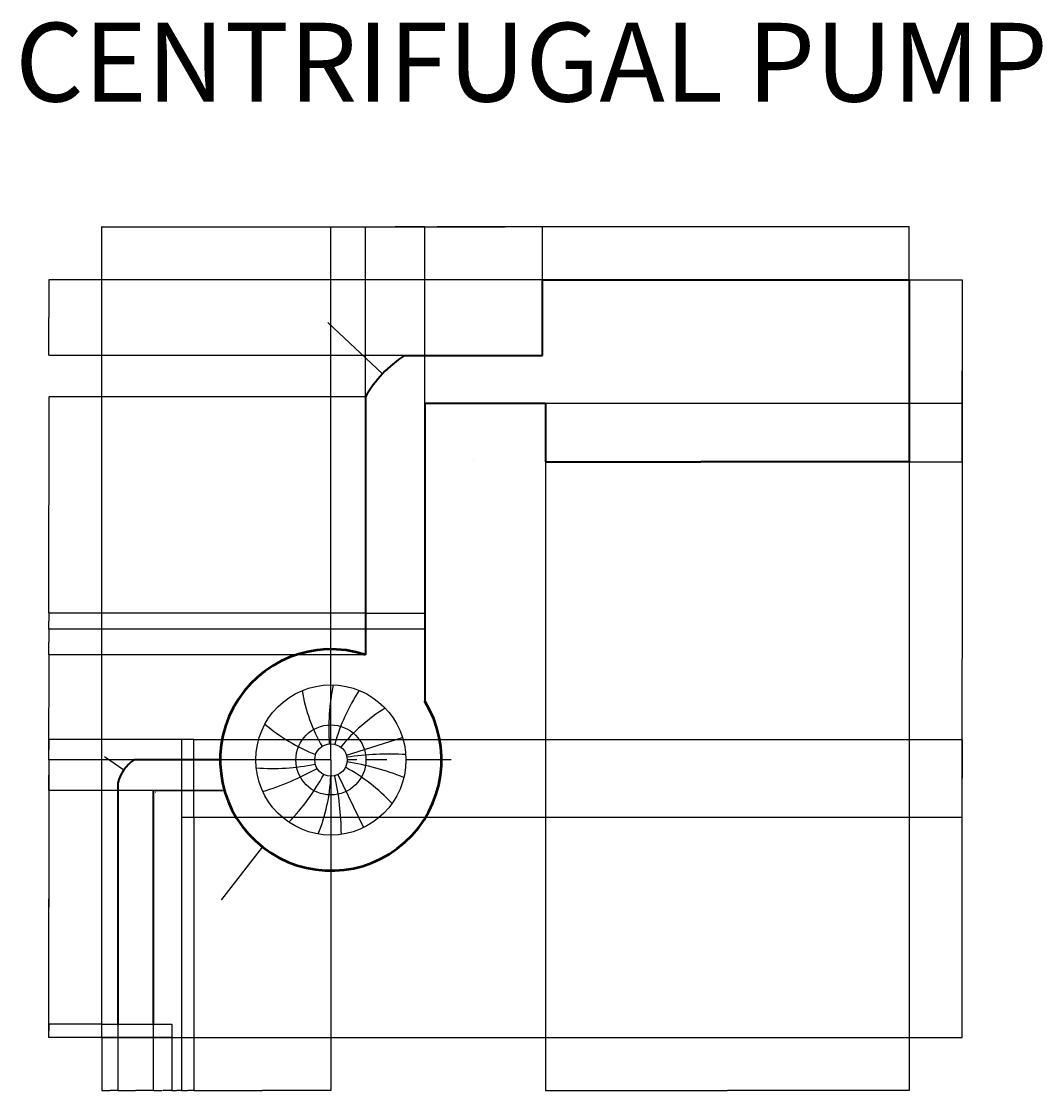
# Model space of a CAD drawing. Units: millimetres. Extents: x 1905 to 3850, y 1033 to 3069.
import ezdxf

# ---------------------------------------------------------------- set-up
doc = ezdxf.new("R2010")
doc.units = ezdxf.units.MM
for name, color, linetype, lineweight in [('A-ANNO-DIMS', 2, 'Continuous', 18), ('M-ANNO-TEXT', 7, 'Continuous', 25), ('M-EQPM-CASG', 7, 'Continuous', 50), ('M-EQPM-IMPL', 4, 'Continuous', 25), ('P-EQPM-TANK', 5, 'Continuous', 35), ('P-PIPE', 3, 'Continuous', 35), ('P-PIPE-FLNG', 6, 'Continuous', 25)]:
    doc.layers.add(name, color=color, linetype=linetype, lineweight=lineweight)
doc.styles.get("Standard").update_dxf_attribs({"font": 'arial.ttf'})
doc.dimstyles.get("Standard").update_dxf_attribs({"dimtxt": 0.18, "dimasz": 0.18, "dimexe": 0.18, "dimexo": 0.0625, "dimgap": 0.09, "dimtad": 0, "dimtih": 1, "dimtoh": 1, "dimdec": 4, "dimzin": 0, "dimdsep": 46, "dimtxsty": 'Standard', "dimcen": 0.09, "dimadec": 0, "dimazin": 0, "dimtfac": 1, "dimtdec": 4, "dimtofl": 0, "dimtmove": 0, "dimatfit": 3, "dimfxl": 1, "dimtolj": 1, "dimtzin": 0, "dimarcsym": 0})

# ---------------------------------------------------------------- blocks, each defined once
blk = doc.blocks.new('*D1')
at = {"layer": 'A-ANNO-DIMS', "color": 0, "lineweight": -2, "transparency": 16777216}
for p, q in [((2058, 1134.2), (2058, 2678.4)), ((2058.1, 2678.2), (2826.3, 2678.2)), ((3595.5, 2678.2), (2827.3, 2678.2)), ((3595.6, 2577.3), (3595.6, 2678.4))]:
    blk.add_line(p, q, dxfattribs=at)
at = {"layer": 'A-ANNO-DIMS', "color": 0, "transparency": 16777216}
for points in [[(2058.1, 2678.3), (2058.1, 2678.2), (2058, 2678.2)], [(3595.5, 2678.3), (3595.5, 2678.2), (3595.6, 2678.2)]]:
    blk.add_solid(points, dxfattribs=at)
at = {"layer": 'Defpoints', "color": 0, "transparency": 16777216}
for p in [(3595.6, 2678.2), (3595.6, 2577.2), (2058, 1134.2)]:
    blk.add_point(p, dxfattribs=at)
at = {"layer": 'A-ANNO-DIMS', "color": 0, "transparency": 16777216, "insert": (2826.8, 2678.2), "char_height": 0.18, "attachment_point": 5}
blk.add_mtext('\\A1;1537.7', dxfattribs=at)
blk = doc.blocks.new('*D2')
at = {"layer": 'A-ANNO-DIMS', "color": 0, "lineweight": -2, "transparency": 16777216}
for p, q in [((3595.7, 2577.2), (3696.8, 2577.2)), ((3696.6, 2577), (3696.6, 1855.9)), ((3696.6, 1134.3), (3696.6, 1855.5)), ((2058, 1134.2), (3696.8, 1134.2))]:
    blk.add_line(p, q, dxfattribs=at)
at = {"layer": 'A-ANNO-DIMS', "color": 0, "transparency": 16777216}
for points in [[(3696.6, 2577), (3696.7, 2577), (3696.6, 2577.2)], [(3696.6, 1134.3), (3696.7, 1134.3), (3696.6, 1134.2)]]:
    blk.add_solid(points, dxfattribs=at)
at = {"layer": 'Defpoints', "color": 0, "transparency": 16777216}
for p in [(3595.6, 2577.2), (3696.6, 2577.2), (2058, 1134.2)]:
    blk.add_point(p, dxfattribs=at)
at = {"layer": 'A-ANNO-DIMS', "color": 0, "transparency": 16777216, "insert": (3696.6, 1855.7), "char_height": 0.18, "attachment_point": 5}
blk.add_mtext('\\A1;1443', dxfattribs=at)
blk = doc.blocks.new('*D3')
at = {"layer": 'A-ANNO-DIMS', "color": 0, "lineweight": -2, "transparency": 16777216}
for p, q in [((3595.7, 2577.2), (3696.8, 2577.2)), ((3696.6, 2577), (3696.6, 2404.1)), ((3696.6, 2230.9), (3696.6, 2403.8)), ((3595.7, 2230.7), (3696.8, 2230.7))]:
    blk.add_line(p, q, dxfattribs=at)
at = {"layer": 'A-ANNO-DIMS', "color": 0, "transparency": 16777216}
for points in [[(3696.6, 2577), (3696.7, 2577), (3696.6, 2577.2)], [(3696.6, 2230.9), (3696.7, 2230.9), (3696.6, 2230.7)]]:
    blk.add_solid(points, dxfattribs=at)
at = {"layer": 'Defpoints', "color": 0, "transparency": 16777216}
for p in [(3595.6, 2577.2), (3696.6, 2577.2), (3595.6, 2230.7)]:
    blk.add_point(p, dxfattribs=at)
at = {"layer": 'A-ANNO-DIMS', "color": 0, "transparency": 16777216, "insert": (3696.6, 2404), "char_height": 0.18, "attachment_point": 5}
blk.add_mtext('\\A1;346.5', dxfattribs=at)
blk = doc.blocks.new('*D4')
at = {"layer": 'A-ANNO-DIMS', "color": 0, "lineweight": -2, "transparency": 16777216}
for p, q in [((2559.8, 2354.1), (2559.8, 2678.4)), ((2560, 2678.2), (2615.9, 2678.2)), ((2672.8, 2678.2), (2616.8, 2678.2)), ((2672.9, 2342), (2672.9, 2678.4))]:
    blk.add_line(p, q, dxfattribs=at)
at = {"layer": 'A-ANNO-DIMS', "color": 0, "transparency": 16777216}
for points in [[(2560, 2678.3), (2560, 2678.2), (2559.8, 2678.2)], [(2672.8, 2678.3), (2672.8, 2678.2), (2672.9, 2678.2)]]:
    blk.add_solid(points, dxfattribs=at)
at = {"layer": 'Defpoints', "color": 0, "transparency": 16777216}
for p in [(2672.9, 2678.2), (2559.8, 2354), (2672.9, 2341.9)]:
    blk.add_point(p, dxfattribs=at)
at = {"layer": 'A-ANNO-DIMS', "color": 0, "transparency": 16777216, "insert": (2616.4, 2678.2), "char_height": 0.18, "attachment_point": 5}
blk.add_mtext('\\A1;113.14', dxfattribs=at)
blk = doc.blocks.new('*D5')
at = {"layer": 'A-ANNO-DIMS', "color": 0, "lineweight": -2, "transparency": 16777216}
for p, q in [((2088.4, 1157.8), (2088.4, 1033)), ((2058, 1134.1), (2058, 1033)), ((2058.1, 1033.2), (2072.8, 1033.2)), ((2088.2, 1033.2), (2073.6, 1033.2))]:
    blk.add_line(p, q, dxfattribs=at)
at = {"layer": 'A-ANNO-DIMS', "color": 0, "transparency": 16777216}
for points in [[(2058.1, 1033.2), (2058.1, 1033.1), (2058, 1033.2)], [(2088.2, 1033.2), (2088.2, 1033.1), (2088.4, 1033.2)]]:
    blk.add_solid(points, dxfattribs=at)
at = {"layer": 'Defpoints', "color": 0, "transparency": 16777216}
for p in [(2088.4, 1157.9), (2058, 1134.2), (2088.4, 1033.2)]:
    blk.add_point(p, dxfattribs=at)
at = {"layer": 'A-ANNO-DIMS', "color": 0, "transparency": 16777216, "insert": (2073.2, 1033.2), "char_height": 0.18, "attachment_point": 5}
blk.add_mtext('\\A1;30.45', dxfattribs=at)
blk = doc.blocks.new('*D6')
at = {"layer": 'A-ANNO-DIMS', "color": 0, "lineweight": -2, "transparency": 16777216}
for p, q in [((2088.4, 1157.8), (2088.4, 1033)), ((2155.9, 1157.8), (2155.9, 1033)), ((2088.6, 1033.2), (2121.8, 1033.2)), ((2155.7, 1033.2), (2122.5, 1033.2))]:
    blk.add_line(p, q, dxfattribs=at)
at = {"layer": 'A-ANNO-DIMS', "color": 0, "transparency": 16777216}
for points in [[(2088.6, 1033.2), (2088.6, 1033.1), (2088.4, 1033.2)], [(2155.7, 1033.2), (2155.7, 1033.1), (2155.9, 1033.2)]]:
    blk.add_solid(points, dxfattribs=at)
at = {"layer": 'Defpoints', "color": 0, "transparency": 16777216}
for p in [(2088.4, 1157.9), (2155.9, 1157.9), (2155.9, 1033.2)]:
    blk.add_point(p, dxfattribs=at)
at = {"layer": 'A-ANNO-DIMS', "color": 0, "transparency": 16777216, "insert": (2122.1, 1033.2), "char_height": 0.18, "attachment_point": 5}
blk.add_mtext('\\A1;67.46', dxfattribs=at)
blk = doc.blocks.new('*D7')
at = {"layer": 'A-ANNO-DIMS', "color": 0, "lineweight": -2, "transparency": 16777216}
for p, q in [((2155.9, 1157.8), (2155.9, 1033)), ((2191.2, 1134.1), (2191.2, 1033)), ((2156.1, 1033.2), (2173.1, 1033.2)), ((2191, 1033.2), (2174, 1033.2))]:
    blk.add_line(p, q, dxfattribs=at)
at = {"layer": 'A-ANNO-DIMS', "color": 0, "transparency": 16777216}
for points in [[(2156.1, 1033.2), (2156.1, 1033.1), (2155.9, 1033.2)], [(2191, 1033.2), (2191, 1033.1), (2191.2, 1033.2)]]:
    blk.add_solid(points, dxfattribs=at)
at = {"layer": 'Defpoints', "color": 0, "transparency": 16777216}
for p in [(2155.9, 1157.9), (2191.2, 1134.2), (2191.2, 1033.2)]:
    blk.add_point(p, dxfattribs=at)
at = {"layer": 'A-ANNO-DIMS', "color": 0, "transparency": 16777216, "insert": (2173.5, 1033.2), "char_height": 0.18, "attachment_point": 5}
blk.add_mtext('\\A1;35.306', dxfattribs=at)
blk = doc.blocks.new('*D8')
at = {"layer": 'A-ANNO-DIMS', "color": 0, "lineweight": -2, "transparency": 16777216}
for p, q in [((2209.4, 1553.6), (2209.4, 1033)), ((2191.2, 1134.1), (2191.2, 1033)), ((2191.4, 1033.2), (2199.9, 1033.2)), ((2209.2, 1033.2), (2200.7, 1033.2))]:
    blk.add_line(p, q, dxfattribs=at)
at = {"layer": 'A-ANNO-DIMS', "color": 0, "transparency": 16777216}
for points in [[(2191.4, 1033.2), (2191.4, 1033.1), (2191.2, 1033.2)], [(2209.2, 1033.2), (2209.2, 1033.1), (2209.4, 1033.2)]]:
    blk.add_solid(points, dxfattribs=at)
at = {"layer": 'Defpoints', "color": 0, "transparency": 16777216}
for p in [(2209.4, 1553.6), (2191.2, 1134.2), (2209.4, 1033.2)]:
    blk.add_point(p, dxfattribs=at)
at = {"layer": 'A-ANNO-DIMS', "color": 0, "transparency": 16777216, "insert": (2200.3, 1033.2), "char_height": 0.18, "attachment_point": 5}
blk.add_mtext('\\A1;18.25', dxfattribs=at)
blk = doc.blocks.new('*D9')
at = {"layer": 'A-ANNO-DIMS', "color": 0, "lineweight": -2, "transparency": 16777216}
for p, q in [((2209.4, 1553.6), (2209.4, 1033)), ((2233.2, 1553.6), (2233.2, 1033)), ((2209.6, 1033.2), (2220.8, 1033.2)), ((2233, 1033.2), (2221.8, 1033.2))]:
    blk.add_line(p, q, dxfattribs=at)
at = {"layer": 'A-ANNO-DIMS', "color": 0, "transparency": 16777216}
for points in [[(2209.6, 1033.2), (2209.6, 1033.1), (2209.4, 1033.2)], [(2233, 1033.2), (2233, 1033.1), (2233.2, 1033.2)]]:
    blk.add_solid(points, dxfattribs=at)
at = {"layer": 'Defpoints', "color": 0, "transparency": 16777216}
for p in [(2209.4, 1553.6), (2233.2, 1553.6), (2233.2, 1033.2)]:
    blk.add_point(p, dxfattribs=at)
at = {"layer": 'A-ANNO-DIMS', "color": 0, "transparency": 16777216, "insert": (2221.3, 1033.2), "char_height": 0.18, "attachment_point": 5}
blk.add_mtext('\\A1;23.723', dxfattribs=at)
blk = doc.blocks.new('*D10')
at = {"layer": 'A-ANNO-DIMS', "color": 0, "lineweight": -2, "transparency": 16777216}
for p, q in [((2494.2, 1662.6), (2494.2, 1033)), ((2233.2, 1553.6), (2233.2, 1033)), ((2233.3, 1033.2), (2363.2, 1033.2)), ((2494, 1033.2), (2364.1, 1033.2))]:
    blk.add_line(p, q, dxfattribs=at)
at = {"layer": 'A-ANNO-DIMS', "color": 0, "transparency": 16777216}
for points in [[(2233.3, 1033.2), (2233.3, 1033.1), (2233.2, 1033.2)], [(2494, 1033.2), (2494, 1033.1), (2494.2, 1033.2)]]:
    blk.add_solid(points, dxfattribs=at)
at = {"layer": 'Defpoints', "color": 0, "transparency": 16777216}
for p in [(2494.2, 1662.7), (2233.2, 1553.6), (2494.2, 1033.2)]:
    blk.add_point(p, dxfattribs=at)
at = {"layer": 'A-ANNO-DIMS', "color": 0, "transparency": 16777216, "insert": (2363.7, 1033.2), "char_height": 0.18, "attachment_point": 5}
blk.add_mtext('\\A1;261.05', dxfattribs=at)
blk = doc.blocks.new('*D11')
at = {"layer": 'A-ANNO-DIMS', "color": 0, "lineweight": -2, "transparency": 16777216}
for p, q in [((2057.9, 1159.7), (1956.8, 1159.7)), ((1957, 1159.5), (1957, 1147.1)), ((1957, 1134.3), (1957, 1146.7)), ((2057.9, 1134.2), (1956.8, 1134.2))]:
    blk.add_line(p, q, dxfattribs=at)
at = {"layer": 'A-ANNO-DIMS', "color": 0, "transparency": 16777216}
for points in [[(1956.9, 1159.5), (1957, 1159.5), (1957, 1159.7)], [(1956.9, 1134.3), (1957, 1134.3), (1957, 1134.2)]]:
    blk.add_solid(points, dxfattribs=at)
at = {"layer": 'Defpoints', "color": 0, "transparency": 16777216}
for p in [(1957, 1159.7), (2058, 1159.7), (2058, 1134.2)]:
    blk.add_point(p, dxfattribs=at)
at = {"layer": 'A-ANNO-DIMS', "color": 0, "transparency": 16777216, "insert": (1957, 1146.9), "char_height": 0.18, "attachment_point": 5}
blk.add_mtext('\\A1;25.534', dxfattribs=at)
blk = doc.blocks.new('*D12')
at = {"layer": 'A-ANNO-DIMS', "color": 0, "lineweight": -2, "transparency": 16777216}
for p, q in [((2155.8, 1604.7), (1956.8, 1604.7)), ((1957, 1604.5), (1957, 1382.4)), ((1957, 1159.9), (1957, 1382)), ((2057.9, 1159.7), (1956.8, 1159.7))]:
    blk.add_line(p, q, dxfattribs=at)
at = {"layer": 'A-ANNO-DIMS', "color": 0, "transparency": 16777216}
for points in [[(1956.9, 1604.5), (1957, 1604.5), (1957, 1604.7)], [(1956.9, 1159.9), (1957, 1159.9), (1957, 1159.7)]]:
    blk.add_solid(points, dxfattribs=at)
at = {"layer": 'Defpoints', "color": 0, "transparency": 16777216}
for p in [(1957, 1604.7), (2155.9, 1604.7), (2058, 1159.7)]:
    blk.add_point(p, dxfattribs=at)
at = {"layer": 'A-ANNO-DIMS', "color": 0, "transparency": 16777216, "insert": (1957, 1382.2), "char_height": 0.18, "attachment_point": 5}
blk.add_mtext('\\A1;445', dxfattribs=at)
blk = doc.blocks.new('*D13')
at = {"layer": 'A-ANNO-DIMS', "color": 0, "lineweight": -2, "transparency": 16777216}
for p, q in [((2119.5, 1663.1), (1956.8, 1663.1)), ((1957, 1662.9), (1957, 1634.1)), ((1957, 1604.9), (1957, 1633.7)), ((2155.8, 1604.7), (1956.8, 1604.7))]:
    blk.add_line(p, q, dxfattribs=at)
at = {"layer": 'A-ANNO-DIMS', "color": 0, "transparency": 16777216}
for points in [[(1956.9, 1662.9), (1957, 1662.9), (1957, 1663.1)], [(1956.9, 1604.9), (1957, 1604.9), (1957, 1604.7)]]:
    blk.add_solid(points, dxfattribs=at)
at = {"layer": 'Defpoints', "color": 0, "transparency": 16777216}
for p in [(1957, 1663.1), (2119.5, 1663.1), (2155.9, 1604.7)]:
    blk.add_point(p, dxfattribs=at)
at = {"layer": 'A-ANNO-DIMS', "color": 0, "transparency": 16777216, "insert": (1957, 1633.9), "char_height": 0.18, "attachment_point": 5}
blk.add_mtext('\\A1;58.36', dxfattribs=at)
blk = doc.blocks.new('*D14')
at = {"layer": 'A-ANNO-DIMS', "color": 0, "lineweight": -2, "transparency": 16777216}
for p, q in [((2209.4, 1701.4), (1956.8, 1701.4)), ((1957, 1701.2), (1957, 1682.4)), ((1957, 1663.3), (1957, 1682)), ((2119.5, 1663.1), (1956.8, 1663.1))]:
    blk.add_line(p, q, dxfattribs=at)
at = {"layer": 'A-ANNO-DIMS', "color": 0, "transparency": 16777216}
for points in [[(1956.9, 1701.2), (1957, 1701.2), (1957, 1701.4)], [(1956.9, 1663.3), (1957, 1663.3), (1957, 1663.1)]]:
    blk.add_solid(points, dxfattribs=at)
at = {"layer": 'Defpoints', "color": 0, "transparency": 16777216}
for p in [(1957, 1701.4), (2209.4, 1701.4), (2119.5, 1663.1)]:
    blk.add_point(p, dxfattribs=at)
at = {"layer": 'A-ANNO-DIMS', "color": 0, "transparency": 16777216, "insert": (1957, 1682.2), "char_height": 0.18, "attachment_point": 5}
blk.add_mtext('\\A1;38.3', dxfattribs=at)
blk = doc.blocks.new('*D15')
at = {"layer": 'A-ANNO-DIMS', "color": 0, "lineweight": -2, "transparency": 16777216}
for p, q in [((2233.2, 1701.4), (3696.8, 1701.4)), ((3696.6, 1701.2), (3696.6, 1627.7)), ((3696.6, 1553.8), (3696.6, 1627.3)), ((2233.2, 1553.6), (3696.8, 1553.6))]:
    blk.add_line(p, q, dxfattribs=at)
at = {"layer": 'A-ANNO-DIMS', "color": 0, "transparency": 16777216}
for points in [[(3696.6, 1701.2), (3696.7, 1701.2), (3696.6, 1701.4)], [(3696.6, 1553.8), (3696.7, 1553.8), (3696.6, 1553.6)]]:
    blk.add_solid(points, dxfattribs=at)
at = {"layer": 'Defpoints', "color": 0, "transparency": 16777216}
for p in [(2233.2, 1701.4), (3696.6, 1701.4), (2233.2, 1553.6)]:
    blk.add_point(p, dxfattribs=at)
at = {"layer": 'A-ANNO-DIMS', "color": 0, "transparency": 16777216, "insert": (3696.6, 1627.5), "char_height": 0.18, "attachment_point": 5}
blk.add_mtext('\\A1;147.73', dxfattribs=at)
blk = doc.blocks.new('*D16')
at = {"layer": 'A-ANNO-DIMS', "color": 0, "lineweight": -2, "transparency": 16777216}
for p, q in [((2494.1, 1662.7), (1956.8, 1662.7)), ((1957, 1662.5), (1957, 1398.6)), ((1957, 1134.3), (1957, 1398.2)), ((2057.9, 1134.2), (1956.8, 1134.2))]:
    blk.add_line(p, q, dxfattribs=at)
at = {"layer": 'A-ANNO-DIMS', "color": 0, "transparency": 16777216}
for points in [[(1956.9, 1662.5), (1957, 1662.5), (1957, 1662.7)], [(1956.9, 1134.3), (1957, 1134.3), (1957, 1134.2)]]:
    blk.add_solid(points, dxfattribs=at)
at = {"layer": 'Defpoints', "color": 0, "transparency": 16777216}
for p in [(1957, 1662.7), (2494.2, 1662.7), (2058, 1134.2)]:
    blk.add_point(p, dxfattribs=at)
at = {"layer": 'A-ANNO-DIMS', "color": 0, "transparency": 16777216, "insert": (1957, 1398.4), "char_height": 0.18, "attachment_point": 5}
blk.add_mtext('\\A1;528.5', dxfattribs=at)
blk = doc.blocks.new('*D17')
at = {"layer": 'A-ANNO-DIMS', "color": 0, "lineweight": -2, "transparency": 16777216}
for p, q in [((2559.7, 1863), (1956.8, 1863)), ((1957, 1862.9), (1957, 1763)), ((1957, 1662.8), (1957, 1762.7)), ((2494.1, 1662.7), (1956.8, 1662.7))]:
    blk.add_line(p, q, dxfattribs=at)
at = {"layer": 'A-ANNO-DIMS', "color": 0, "transparency": 16777216}
for points in [[(1956.9, 1862.9), (1957, 1862.9), (1957, 1863)], [(1956.9, 1662.8), (1957, 1662.8), (1957, 1662.7)]]:
    blk.add_solid(points, dxfattribs=at)
at = {"layer": 'Defpoints', "color": 0, "transparency": 16777216}
for p in [(1957, 1863), (2559.8, 1863), (2494.2, 1662.7)]:
    blk.add_point(p, dxfattribs=at)
at = {"layer": 'A-ANNO-DIMS', "color": 0, "transparency": 16777216, "insert": (1957, 1762.8), "char_height": 0.18, "attachment_point": 5}
blk.add_mtext('\\A1;200.4', dxfattribs=at)
blk = doc.blocks.new('*D18')
at = {"layer": 'A-ANNO-DIMS', "color": 0, "lineweight": -2, "transparency": 16777216}
for p, q in [((2559.7, 1911.5), (1956.8, 1911.5)), ((1957, 1911.3), (1957, 1887.5)), ((1957, 1863.2), (1957, 1887.1)), ((2559.7, 1863), (1956.8, 1863))]:
    blk.add_line(p, q, dxfattribs=at)
at = {"layer": 'A-ANNO-DIMS', "color": 0, "transparency": 16777216}
for points in [[(1956.9, 1911.3), (1957, 1911.3), (1957, 1911.5)], [(1956.9, 1863.2), (1957, 1863.2), (1957, 1863)]]:
    blk.add_solid(points, dxfattribs=at)
at = {"layer": 'Defpoints', "color": 0, "transparency": 16777216}
for p in [(1957, 1911.5), (2559.8, 1911.5), (2559.8, 1863)]:
    blk.add_point(p, dxfattribs=at)
at = {"layer": 'A-ANNO-DIMS', "color": 0, "transparency": 16777216, "insert": (1957, 1887.3), "char_height": 0.18, "attachment_point": 5}
blk.add_mtext('\\A1;48.475', dxfattribs=at)
blk = doc.blocks.new('*D19')
at = {"layer": 'A-ANNO-DIMS', "color": 0, "lineweight": -2, "transparency": 16777216}
for p, q in [((2559.7, 1942.5), (1956.8, 1942.5)), ((1957, 1942.3), (1957, 1927.2)), ((1957, 1911.7), (1957, 1926.8)), ((2559.7, 1911.5), (1956.8, 1911.5))]:
    blk.add_line(p, q, dxfattribs=at)
at = {"layer": 'A-ANNO-DIMS', "color": 0, "transparency": 16777216}
for points in [[(1956.9, 1942.3), (1957, 1942.3), (1957, 1942.5)], [(1956.9, 1911.7), (1957, 1911.7), (1957, 1911.5)]]:
    blk.add_solid(points, dxfattribs=at)
at = {"layer": 'Defpoints', "color": 0, "transparency": 16777216}
for p in [(1957, 1942.5), (2559.8, 1942.5), (2559.8, 1911.5)]:
    blk.add_point(p, dxfattribs=at)
at = {"layer": 'A-ANNO-DIMS', "color": 0, "transparency": 16777216, "insert": (1957, 1927), "char_height": 0.18, "attachment_point": 5}
blk.add_mtext('\\A1;31.006', dxfattribs=at)
blk = doc.blocks.new('*D20')
at = {"layer": 'A-ANNO-DIMS', "color": 0, "lineweight": -2, "transparency": 16777216}
for p, q in [((2559.7, 2354), (1956.8, 2354)), ((1957, 2353.9), (1957, 2148.5)), ((1957, 1942.7), (1957, 2148.1)), ((2559.7, 1942.5), (1956.8, 1942.5))]:
    blk.add_line(p, q, dxfattribs=at)
at = {"layer": 'A-ANNO-DIMS', "color": 0, "transparency": 16777216}
for points in [[(1956.9, 2353.9), (1957, 2353.9), (1957, 2354)], [(1956.9, 1942.7), (1957, 1942.7), (1957, 1942.5)]]:
    blk.add_solid(points, dxfattribs=at)
at = {"layer": 'Defpoints', "color": 0, "transparency": 16777216}
for p in [(1957, 2354), (2559.8, 2354), (2559.8, 1942.5)]:
    blk.add_point(p, dxfattribs=at)
at = {"layer": 'A-ANNO-DIMS', "color": 0, "transparency": 16777216, "insert": (1957, 2148.3), "char_height": 0.18, "attachment_point": 5}
blk.add_mtext('\\A1;411.5', dxfattribs=at)
blk = doc.blocks.new('*D21')
at = {"layer": 'A-ANNO-DIMS', "color": 0, "lineweight": -2, "transparency": 16777216}
for p, q in [((2494.2, 1662.7), (2494.2, 2678.4)), ((2494.4, 2678.2), (2695.4, 2678.2)), ((2897.4, 2678.2), (2696.3, 2678.2)), ((2897.5, 2577.3), (2897.5, 2678.4))]:
    blk.add_line(p, q, dxfattribs=at)
at = {"layer": 'A-ANNO-DIMS', "color": 0, "transparency": 16777216}
for points in [[(2494.4, 2678.3), (2494.4, 2678.2), (2494.2, 2678.2)], [(2897.4, 2678.3), (2897.4, 2678.2), (2897.5, 2678.2)]]:
    blk.add_solid(points, dxfattribs=at)
at = {"layer": 'Defpoints', "color": 0, "transparency": 16777216}
for p in [(2897.5, 2678.2), (2897.5, 2577.2), (2494.2, 1662.7)]:
    blk.add_point(p, dxfattribs=at)
at = {"layer": 'A-ANNO-DIMS', "color": 0, "transparency": 16777216, "insert": (2695.9, 2678.2), "char_height": 0.18, "attachment_point": 5}
blk.add_mtext('\\A1;403.34', dxfattribs=at)
blk = doc.blocks.new('*D22')
at = {"layer": 'A-ANNO-DIMS', "color": 0, "lineweight": -2, "transparency": 16777216}
for p, q in [((2903, 2230.6), (2903, 1033)), ((3595.6, 2230.6), (3595.6, 1033)), ((2903.2, 1033.2), (3248.9, 1033.2)), ((3595.5, 1033.2), (3249.7, 1033.2))]:
    blk.add_line(p, q, dxfattribs=at)
at = {"layer": 'A-ANNO-DIMS', "color": 0, "transparency": 16777216}
for points in [[(2903.2, 1033.2), (2903.2, 1033.1), (2903, 1033.2)], [(3595.5, 1033.2), (3595.5, 1033.1), (3595.6, 1033.2)]]:
    blk.add_solid(points, dxfattribs=at)
at = {"layer": 'Defpoints', "color": 0, "transparency": 16777216}
for p in [(2903, 2230.7), (3595.6, 2230.7), (3595.6, 1033.2)]:
    blk.add_point(p, dxfattribs=at)
at = {"layer": 'A-ANNO-DIMS', "color": 0, "transparency": 16777216, "insert": (3249.3, 1033.2), "char_height": 0.18, "attachment_point": 5}
blk.add_mtext('\\A1;692.6', dxfattribs=at)
blk = doc.blocks.new('*D23')
at = {"layer": 'A-ANNO-DIMS', "color": 0, "lineweight": -2, "transparency": 16777216}
for p, q in [((2897.5, 2577.2), (1956.8, 2577.2)), ((1957, 2577), (1957, 2505.4)), ((1957, 2433.3), (1957, 2505)), ((2897.5, 2433.1), (1956.8, 2433.1))]:
    blk.add_line(p, q, dxfattribs=at)
at = {"layer": 'A-ANNO-DIMS', "color": 0, "transparency": 16777216}
for points in [[(1956.9, 2577), (1957, 2577), (1957, 2577.2)], [(1956.9, 2433.3), (1957, 2433.3), (1957, 2433.1)]]:
    blk.add_solid(points, dxfattribs=at)
at = {"layer": 'Defpoints', "color": 0, "transparency": 16777216}
for p in [(1957, 2577.2), (2897.5, 2577.2), (2897.5, 2433.1)]:
    blk.add_point(p, dxfattribs=at)
at = {"layer": 'A-ANNO-DIMS', "color": 0, "transparency": 16777216, "insert": (1957, 2505.2), "char_height": 0.18, "attachment_point": 5}
blk.add_mtext('\\A1;144.09', dxfattribs=at)
blk = doc.blocks.new('*D24')
at = {"layer": 'A-ANNO-DIMS', "color": 0, "lineweight": -2, "transparency": 16777216}
for p, q in [((2903.1, 2341.9), (3696.8, 2341.9)), ((3696.6, 2341.8), (3696.6, 2286.5)), ((3696.6, 2230.9), (3696.6, 2286.1)), ((2903.1, 2230.7), (3696.8, 2230.7))]:
    blk.add_line(p, q, dxfattribs=at)
at = {"layer": 'A-ANNO-DIMS', "color": 0, "transparency": 16777216}
for points in [[(3696.6, 2341.8), (3696.7, 2341.8), (3696.6, 2341.9)], [(3696.6, 2230.9), (3696.7, 2230.9), (3696.6, 2230.7)]]:
    blk.add_solid(points, dxfattribs=at)
at = {"layer": 'Defpoints', "color": 0, "transparency": 16777216}
for p in [(2903, 2341.9), (3696.6, 2341.9), (2903, 2230.7)]:
    blk.add_point(p, dxfattribs=at)
at = {"layer": 'A-ANNO-DIMS', "color": 0, "transparency": 16777216, "insert": (3696.6, 2286.3), "char_height": 0.18, "attachment_point": 5}
blk.add_mtext('\\A1;111.26', dxfattribs=at)
blk = doc.blocks.new('*D25')
at = {"layer": 'A-ANNO-DIMS', "color": 0, "lineweight": -2, "transparency": 16777216}
for p, q in [((2494.1, 1662.7), (2494.3, 1662.7)), ((2494.2, 1662.6), (2494.2, 1662.7)), ((2286.3, 1397), (2364.1, 1496.5)), ((2286.1, 1397), (2286.3, 1397))]:
    blk.add_line(p, q, dxfattribs=at)
at = {"layer": 'A-ANNO-DIMS', "color": 0, "transparency": 16777216}
blk.add_solid([(2364.1, 1496.5), (2364.2, 1496.4), (2364.3, 1496.6)], dxfattribs=at)
at = {"layer": 'Defpoints', "color": 0, "transparency": 16777216}
for p in [(2494.2, 1662.7), (2364.3, 1496.6)]:
    blk.add_point(p, dxfattribs=at)
at = {"layer": 'A-ANNO-DIMS', "color": 0, "transparency": 16777216, "insert": (2285.6, 1397), "char_height": 0.18, "attachment_point": 5}
blk.add_mtext('\\A1;R210.85', dxfattribs=at)
blk = doc.blocks.new('*D26')
at = {"layer": 'A-ANNO-DIMS', "color": 0, "lineweight": -2, "transparency": 16777216}
for p, q in [((2488.2, 2495.8), (2488.4, 2495.8)), ((2488.4, 2495.8), (2592.3, 2398)), ((2765.8, 2234.7), (2766, 2234.7)), ((2765.9, 2234.6), (2765.9, 2234.8))]:
    blk.add_line(p, q, dxfattribs=at)
at = {"layer": 'A-ANNO-DIMS', "color": 0, "transparency": 16777216}
blk.add_solid([(2592.3, 2398), (2592.3, 2398), (2592.5, 2397.9)], dxfattribs=at)
at = {"layer": 'Defpoints', "color": 0, "transparency": 16777216}
for p in [(2592.5, 2397.9), (2765.9, 2234.7)]:
    blk.add_point(p, dxfattribs=at)
at = {"layer": 'A-ANNO-DIMS', "color": 0, "transparency": 16777216, "insert": (2487.7, 2495.8), "char_height": 0.18, "attachment_point": 5}
blk.add_mtext('\\A1;R238.16', dxfattribs=at)
blk = doc.blocks.new('*D27')
at = {"layer": 'A-ANNO-DIMS', "color": 0, "lineweight": -2, "transparency": 16777216}
for p, q in [((2063, 1669.1), (2063.2, 1669.1)), ((2063.2, 1669.1), (2099.6, 1643.8)), ((2160.4, 1601.4), (2160.6, 1601.4)), ((2160.5, 1601.3), (2160.5, 1601.5))]:
    blk.add_line(p, q, dxfattribs=at)
at = {"layer": 'A-ANNO-DIMS', "color": 0, "transparency": 16777216}
blk.add_solid([(2099.6, 1643.8), (2099.5, 1643.8), (2099.7, 1643.7)], dxfattribs=at)
at = {"layer": 'Defpoints', "color": 0, "transparency": 16777216}
for p in [(2099.7, 1643.7), (2160.5, 1601.4)]:
    blk.add_point(p, dxfattribs=at)
at = {"layer": 'A-ANNO-DIMS', "color": 0, "transparency": 16777216, "insert": (2062.6, 1669.1), "char_height": 0.18, "attachment_point": 5}
blk.add_mtext('\\A1;R74.09', dxfattribs=at)
blk = doc.blocks.new('*D28')
at = {"layer": 'A-ANNO-DIMS', "color": 0, "lineweight": -2, "transparency": 16777216}
for p, q in [((2494.1, 1662.7), (2494.3, 1662.7)), ((2494.2, 1662.6), (2494.2, 1662.7)), ((2723, 1662.6), (2637.4, 1662.6))]:
    blk.add_line(p, q, dxfattribs=at)
at = {"layer": 'A-ANNO-DIMS', "color": 0, "transparency": 16777216}
blk.add_solid([(2637.4, 1662.7), (2637.4, 1662.6), (2637.2, 1662.6)], dxfattribs=at)
at = {"layer": 'Defpoints', "color": 0, "transparency": 16777216}
for p in [(2351.2, 1662.7), (2637.2, 1662.6)]:
    blk.add_point(p, dxfattribs=at)
at = {"layer": 'A-ANNO-DIMS', "color": 0, "transparency": 16777216, "insert": (2723.4, 1662.6), "char_height": 0.18, "attachment_point": 5}
blk.add_mtext('\\A1;∅286', dxfattribs=at)
blk = doc.blocks.new('*D29')
at = {"layer": 'A-ANNO-DIMS', "color": 0, "lineweight": -2, "transparency": 16777216}
for p, q in [((2494.1, 1662.7), (2494.3, 1662.7)), ((2494.2, 1662.6), (2494.2, 1662.7)), ((2600.9, 1662.6), (2561.1, 1662.6))]:
    blk.add_line(p, q, dxfattribs=at)
at = {"layer": 'A-ANNO-DIMS', "color": 0, "transparency": 16777216}
blk.add_solid([(2561.1, 1662.7), (2561.1, 1662.6), (2560.9, 1662.6)], dxfattribs=at)
at = {"layer": 'Defpoints', "color": 0, "transparency": 16777216}
for p in [(2427.5, 1662.7), (2560.9, 1662.6)]:
    blk.add_point(p, dxfattribs=at)
at = {"layer": 'A-ANNO-DIMS', "color": 0, "transparency": 16777216, "insert": (2601.4, 1662.6), "char_height": 0.18, "attachment_point": 5}
blk.add_mtext('\\A1;∅133.4', dxfattribs=at)
blk = doc.blocks.new('*D30')
at = {"layer": 'A-ANNO-DIMS', "color": 0, "lineweight": -2, "transparency": 16777216}
for p, q in [((2494.1, 1662.7), (2494.3, 1662.7)), ((2494.2, 1662.6), (2494.2, 1662.7)), ((2543.7, 1662.6), (2525.3, 1662.6))]:
    blk.add_line(p, q, dxfattribs=at)
at = {"layer": 'A-ANNO-DIMS', "color": 0, "transparency": 16777216}
blk.add_solid([(2525.3, 1662.7), (2525.3, 1662.6), (2525.1, 1662.6)], dxfattribs=at)
at = {"layer": 'Defpoints', "color": 0, "transparency": 16777216}
for p in [(2463.3, 1662.7), (2525.1, 1662.6)]:
    blk.add_point(p, dxfattribs=at)
at = {"layer": 'A-ANNO-DIMS', "color": 0, "transparency": 16777216, "insert": (2544.1, 1662.6), "char_height": 0.18, "attachment_point": 5}
blk.add_mtext('\\A1;∅61.82', dxfattribs=at)

msp = doc.modelspace()

# ---------------------------------------------------------------- linework, layer by layer
at = {"layer": 'M-EQPM-CASG'}
msp.add_arc((2494.1971, 1662.654), 210.8533, 71.8718883, 32.0341721, dxfattribs=at)
at = {"layer": 'M-EQPM-IMPL'}
for p, q in [((2523.6847, 1671.92), (2630.6191, 1705.5227)), ((2507.6363, 1634.8194), (2556.3727, 1533.8794)), ((2460.6473, 1605.0053), (2462.7451, 1605.0073))]:
    msp.add_line(p, q, dxfattribs=at)
for radius in [142.9989, 66.7006, 30.9091]:
    msp.add_circle((2494.1971, 1662.654), radius, dxfattribs=at)
for centre, radius, start, end in [((2751.4697, 1847.2274), 316.6332, 189.5553249, 210.061217), ((2917.5712, 1721.8087), 427.4867, 168.6974348, 183.8103587), ((2862.8904, 1589.6214), 375.857, 146.8631447, 164.0824845), ((2784.803, 1461.6328), 353.3572, 121.979131, 140.313756), ((2596.7492, 2001.7862), 354.2987, 229.8897902, 248.1748305), ((2605.9682, 1108.5807), 565.2344, 86.8707736, 98.2714587), ((2384.6286, 2024.1661), 377.7516, 265.0400995, 282.1717405), ((2596.7492, 2001.7862), 354.2987, 253.1749131, 253.1749196), ((2449.3683, 1170.9923), 493.7012, 68.136184, 81.202582), ((2220.3612, 2085.3105), 503.6116, 286.6147809, 299.4218148), ((2123.1954, 1827.6688), 406.0445, 315.7374437, 331.658818), ((2156.3273, 1647.7846), 338.1969, 338.1094871, 357.2816027), ((1969.8752, 1516.7353), 544.2478, 0.4539988, 12.2974744), ((2347.2495, 1332.6684), 361.2258, 43.1633266, 61.0917154)]:
    msp.add_arc(centre, radius, start, end, dxfattribs=at)
at = {"layer": 'P-EQPM-TANK'}
for p, q in [((2897.5403, 2433.1413), (2897.5403, 2577.2266)), ((2897.5403, 2577.2266), (3198.6429, 2577.2266)), ((3198.6429, 2577.2266), (3595.636, 2577.2266)), ((3595.636, 2577.2266), (3595.636, 2230.6924)), ((2903.0149, 2341.9481), (2903.0149, 2230.6924)), ((2903.0149, 2230.6924), (3198.6429, 2230.6924)), ((3595.636, 2230.6924), (3198.6429, 2230.6924))]:
    msp.add_line(p, q, dxfattribs=at)
at = {"layer": 'P-PIPE'}
for p, q in [((2634.2353, 2433.1413), (2897.5403, 2433.1413)), ((2559.8026, 2354.0458), (2559.8026, 1863.0412)), ((2672.9442, 2341.9481), (2672.9442, 1772.5033)), ((2672.9442, 2341.9481), (2758.8506, 2341.9481)), ((2758.8506, 2341.9481), (2903.0149, 2341.9481)), ((2283.3439, 1662.8903), (2119.5128, 1663.0739)), ((2088.417, 1618.409), (2088.417, 1439.177)), ((2155.8737, 1604.7149), (2291.4235, 1604.844)), ((2155.8737, 1604.7149), (2155.8737, 1456.3951)), ((2155.8737, 1456.3951), (2155.8737, 1157.861)), ((2088.417, 1439.177), (2088.417, 1157.861))]:
    msp.add_line(p, q, dxfattribs=at)
for centre, radius, start, end in [((2765.8878, 2234.6799), 238.1582, 123.5589277, 149.9203082), ((2160.5179, 1601.369), 74.0871, 123.6054482, 166.7029639)]:
    msp.add_arc(centre, radius, start, end, dxfattribs=at)
at = {"layer": 'P-PIPE-FLNG'}
for points in [[(2559.8026, 1942.5218), (2672.9442, 1942.5218)], [(2672.9442, 1911.5161), (2559.8026, 1911.5161)]]:
    msp.add_lwpolyline(points, dxfattribs=at)
for points in [[(2233.1519, 1701.3725), (2209.4286, 1701.3725), (2209.4286, 1553.6395), (2233.1519, 1553.6395)], [(2057.9649, 1159.6849), (2191.18, 1159.6849), (2191.18, 1134.1508), (2057.9649, 1134.1508)]]:
    msp.add_lwpolyline(points, close=True, dxfattribs=at)

# ---------------------------------------------------------------- texts
at = {"layer": 'M-ANNO-TEXT', "insert": (1892.7433, 3066.5674), "char_height": 150, "attachment_point": 1}
msp.add_mtext('CENTRIFUGAL PUMP', dxfattribs=at)

# ---------------------------------------------------------------- dimensions: what is measured, and where the dimension line sits
at = {"layer": 'A-ANNO-DIMS'}
for base, p1, p2, override, picture, middle in [((3595.636, 2678.2266), (2057.9649, 1134.1508), (3595.636, 2577.2266), {"dimdec": 1, "dimlfac": 1, "dimrnd": 0, "dimzin": 0, "dimdsep": 46, "dimlunit": 2}, '*D1', (2826.8004, 2678.2266)), ((2897.5403, 2678.2266), (2494.1971, 1662.654), (2897.5403, 2577.2266), {"dimdec": 2, "dimlfac": 1, "dimrnd": 0, "dimzin": 0, "dimdsep": 46, "dimlunit": 2}, '*D21', (2695.8687, 2678.2266)), ((2672.9442, 2678.2266), (2559.8026, 2354.0458), (2672.9442, 2341.9481), {"dimdec": 2, "dimlfac": 1, "dimrnd": 0, "dimzin": 0, "dimdsep": 46, "dimlunit": 2}, '*D4', (2616.3734, 2678.2266)), ((3595.636, 1033.1508), (2903.0149, 2230.6924), (3595.636, 2230.6924), {"dimdec": 1, "dimlfac": 1, "dimrnd": 0, "dimzin": 0, "dimdsep": 46, "dimlunit": 2}, '*D22', (3249.3254, 1033.1508)), ((2494.1971, 1033.1508), (2233.1519, 1553.6395), (2494.1971, 1662.654), {"dimdec": 2, "dimlfac": 1, "dimrnd": 0, "dimzin": 0, "dimdsep": 46, "dimlunit": 2}, '*D10', (2363.6745, 1033.1508)), ((2209.4286, 1033.1508), (2191.18, 1134.1508), (2209.4286, 1553.6395), {"dimdec": 2, "dimlfac": 1, "dimrnd": 0, "dimzin": 0, "dimdsep": 46, "dimlunit": 2}, '*D8', (2200.3043, 1033.1508)), ((2233.1519, 1033.1508), (2209.4286, 1553.6395), (2233.1519, 1553.6395), {"dimdec": 3, "dimlfac": 1, "dimrnd": 0, "dimzin": 0, "dimdsep": 46, "dimlunit": 2}, '*D9', (2221.2903, 1033.1508)), ((2088.417, 1033.1508), (2057.9649, 1134.1508), (2088.417, 1157.861), {"dimdec": 2, "dimlfac": 1, "dimrnd": 0, "dimzin": 0, "dimdsep": 46, "dimlunit": 2}, '*D5', (2073.191, 1033.1508)), ((2155.8737, 1033.1508), (2088.417, 1157.861), (2155.8737, 1157.861), {"dimdec": 2, "dimlfac": 1, "dimrnd": 0, "dimzin": 0, "dimdsep": 46, "dimlunit": 2}, '*D6', (2122.1453, 1033.1508)), ((2191.18, 1033.1508), (2155.8737, 1157.861), (2191.18, 1134.1508), {"dimdec": 3, "dimlfac": 1, "dimrnd": 0, "dimzin": 0, "dimdsep": 46, "dimlunit": 2}, '*D7', (2173.5268, 1033.1508))]:
    dim = msp.add_linear_dim(base=base, p1=p1, p2=p2, dimstyle='Standard', override=override, dxfattribs=at)
    dim.commit()
    dim.dimension.update_dxf_attribs({"geometry": picture, "text_midpoint": middle})
for base, p1, p2, override, picture, middle in [((1956.9649, 2577.2266), (2897.5403, 2433.1413), (2897.5403, 2577.2266), {"dimdec": 2, "dimlfac": 1, "dimrnd": 0, "dimzin": 0, "dimdsep": 46, "dimlunit": 2}, '*D23', (1956.9649, 2505.184)), ((3696.636, 2577.2266), (2057.9649, 1134.1508), (3595.636, 2577.2266), {"dimdec": 0, "dimlfac": 1, "dimrnd": 0, "dimzin": 0, "dimdsep": 46, "dimlunit": 2}, '*D2', (3696.636, 1855.6887)), ((3696.636, 2577.2266), (3595.636, 2230.6924), (3595.636, 2577.2266), {"dimdec": 1, "dimlfac": 1, "dimrnd": 0, "dimzin": 0, "dimdsep": 46, "dimlunit": 2}, '*D3', (3696.636, 2403.9595)), ((1956.9649, 2354.0458), (2559.8026, 1942.5218), (2559.8026, 2354.0458), {"dimdec": 1, "dimlfac": 1, "dimrnd": 0, "dimzin": 0, "dimdsep": 46, "dimlunit": 2}, '*D20', (1956.9649, 2148.2838)), ((3696.636, 2341.9481), (2903.0149, 2230.6924), (2903.0149, 2341.9481), {"dimdec": 2, "dimlfac": 1, "dimrnd": 0, "dimzin": 0, "dimdsep": 46, "dimlunit": 2}, '*D24', (3696.636, 2286.3203)), ((1956.9649, 1942.5218), (2559.8026, 1911.5161), (2559.8026, 1942.5218), {"dimdec": 3, "dimlfac": 1, "dimrnd": 0, "dimzin": 0, "dimdsep": 46, "dimlunit": 2}, '*D19', (1956.9649, 1927.019)), ((1956.9649, 1911.5161), (2559.8026, 1863.0412), (2559.8026, 1911.5161), {"dimdec": 3, "dimlfac": 1, "dimrnd": 0, "dimzin": 0, "dimdsep": 46, "dimlunit": 2}, '*D18', (1956.9649, 1887.2787)), ((1956.9649, 1863.0412), (2494.1971, 1662.654), (2559.8026, 1863.0412), {"dimdec": 1, "dimlfac": 1, "dimrnd": 0, "dimzin": 0, "dimdsep": 46, "dimlunit": 2}, '*D17', (1956.9649, 1762.8476)), ((1956.9649, 1701.3725), (2119.5128, 1663.0739), (2209.4286, 1701.3725), {"dimdec": 1, "dimlfac": 1, "dimrnd": 0, "dimzin": 0, "dimdsep": 46, "dimlunit": 2}, '*D14', (1956.9649, 1682.2232)), ((3696.636, 1701.3725), (2233.1519, 1553.6395), (2233.1519, 1701.3725), {"dimdec": 2, "dimlfac": 1, "dimrnd": 0, "dimzin": 0, "dimdsep": 46, "dimlunit": 2}, '*D15', (3696.636, 1627.506)), ((1956.9649, 1663.0739), (2155.8737, 1604.7149), (2119.5128, 1663.0739), {"dimdec": 2, "dimlfac": 1, "dimrnd": 0, "dimzin": 0, "dimdsep": 46, "dimlunit": 2}, '*D13', (1956.9649, 1633.8944)), ((1956.9649, 1662.654), (2057.9649, 1134.1508), (2494.1971, 1662.654), {"dimdec": 1, "dimlfac": 1, "dimrnd": 0, "dimzin": 0, "dimdsep": 46, "dimlunit": 2}, '*D16', (1956.9649, 1398.4024)), ((1956.9649, 1604.7149), (2057.9649, 1159.6849), (2155.8737, 1604.7149), {"dimdec": 0, "dimlfac": 1, "dimrnd": 0, "dimzin": 0, "dimdsep": 46, "dimlunit": 2}, '*D12', (1956.9649, 1382.1999)), ((1956.9649, 1159.6849), (2057.9649, 1134.1508), (2057.9649, 1159.6849), {"dimdec": 3, "dimlfac": 1, "dimrnd": 0, "dimzin": 0, "dimdsep": 46, "dimlunit": 2}, '*D11', (1956.9649, 1146.9178))]:
    dim = msp.add_linear_dim(base=base, p1=p1, p2=p2, angle=90, dimstyle='Standard', override=override, dxfattribs=at)
    dim.commit()
    dim.dimension.update_dxf_attribs({"geometry": picture, "text_midpoint": middle})
for center, mpoint, picture, middle in [((2765.8878, 2234.6799), (2592.4533, 2397.8969), '*D26', (2487.6629, 2495.8271)), ((2160.5179, 1601.369), (2099.7101, 1643.693), '*D27', (2062.5654, 1669.0873)), ((2494.1971, 1662.654), (2364.2516, 1496.602), '*D25', (2285.5538, 1396.9708))]:
    dim = msp.add_radius_dim(center=center, mpoint=mpoint, dimstyle='Standard', override={"dimdec": 2, "dimlfac": 1, "dimrnd": 0, "dimzin": 0, "dimdsep": 46, "dimlunit": 2}, dxfattribs=at)
    dim.commit()
    dim.dimension.update_dxf_attribs({"geometry": picture, "text_midpoint": middle, "dimtype": 164})
for p1, p2, override, picture, middle in [((2351.1982, 1662.658), (2637.196, 1662.65), {"dimdec": 0, "dimlfac": 1, "dimrnd": 0, "dimzin": 0, "dimdsep": 46, "dimlunit": 2}, '*D28', (2722.9954, 1662.6476)), ((2427.4965, 1662.658), (2560.8977, 1662.65), {"dimdec": 1, "dimlfac": 1, "dimrnd": 0, "dimzin": 0, "dimdsep": 46, "dimlunit": 2}, '*D29', (2600.9181, 1662.6476)), ((2463.288, 1662.658), (2525.1063, 1662.65), {"dimdec": 2, "dimlfac": 1, "dimrnd": 0, "dimzin": 0, "dimdsep": 46, "dimlunit": 2}, '*D30', (2543.6517, 1662.6476))]:
    dim = msp.add_diameter_dim_2p(p1=p1, p2=p2, dimstyle='Standard', override=override, dxfattribs=at)
    dim.commit()
    dim.dimension.update_dxf_attribs({"geometry": picture, "text_midpoint": middle, "dimtype": 163})

doc.saveas('drawing.dxf')
